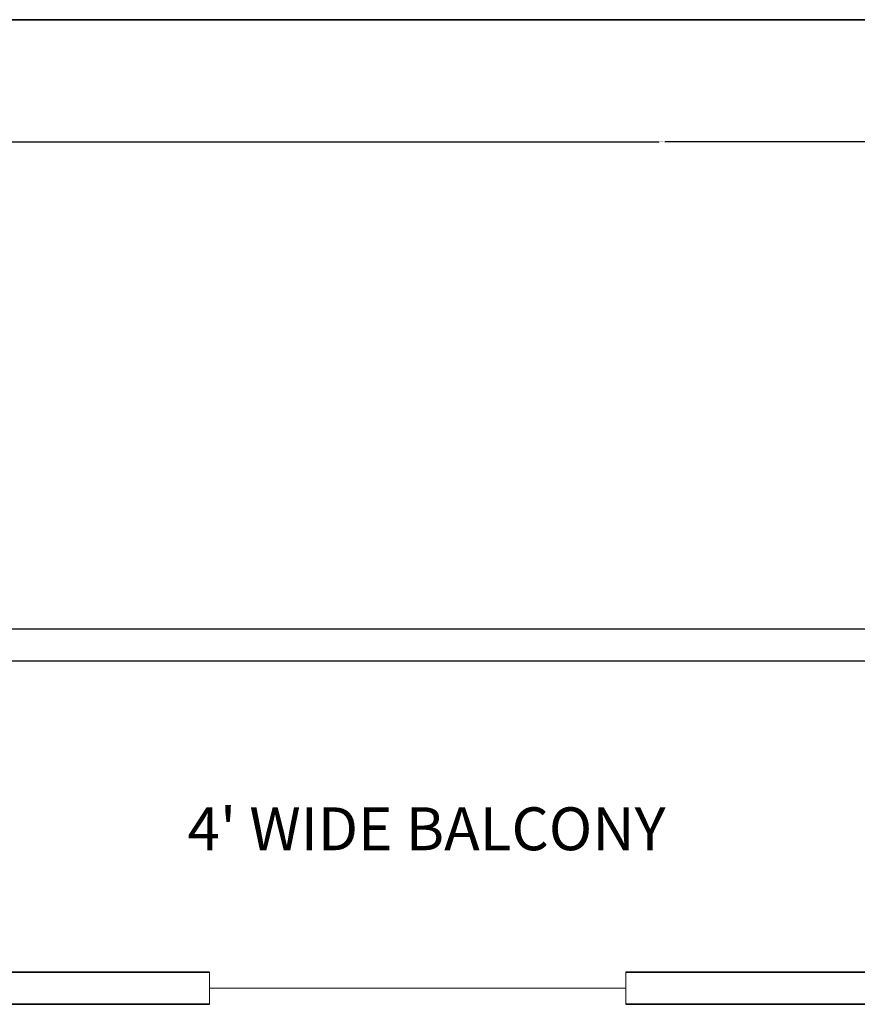
# Model space of a CAD drawing. Units: inches. Extents: x 1088 to 1703, y 668 to 1875.
# Tile 23 of 45: x 1319 to 1436, y 1737 to 1875. Entities that reach past the tile are written whole.
import ezdxf

# ---------------------------------------------------------------- set-up
doc = ezdxf.new("R2010")
doc.units = ezdxf.units.IN
for name, color, linetype, lineweight in [('A-ANNO-DIMS', 2, 'Continuous', 18), ('A-ANNO-TTLB', 7, 'Continuous', 35), ('A-AREA-IDEN', 7, 'Continuous', 18), ('A-DOOR', 4, 'Continuous', 18), ('A-FLOR-HRAL', 7, 'Continuous', 25), ('A-WALL', 7, 'Continuous', 35)]:
    doc.layers.add(name, color=color, linetype=linetype, lineweight=lineweight)
doc.styles.get("Standard").update_dxf_attribs({"font": 'arial.ttf'})
doc.dimstyles.get("Standard").update_dxf_attribs({"dimtxt": 0.18, "dimasz": 0.18, "dimexe": 0.18, "dimexo": 0.0625, "dimgap": 0.09, "dimtad": 0, "dimtih": 1, "dimtoh": 1, "dimdec": 4, "dimzin": 0, "dimdsep": 46, "dimtxsty": 'Standard', "dimcen": 0.09, "dimadec": 0, "dimazin": 0, "dimtfac": 1, "dimtdec": 4, "dimtofl": 0, "dimtmove": 0, "dimatfit": 3, "dimfxl": 1, "dimtolj": 1, "dimtzin": 0, "dimarcsym": 0})

# ---------------------------------------------------------------- blocks, each defined once
blk = doc.blocks.new('*D28')
at = {"layer": 'A-ANNO-DIMS', "color": 0, "lineweight": -2, "transparency": 16777216}
for p, q in [((1170.34, 1803.62), (1170.34, 1857.79)), ((1170.52, 1857.61), (1408.15, 1857.61)), ((1646.56, 1857.61), (1408.94, 1857.61)), ((1646.74, 1745.55), (1646.74, 1857.79))]:
    blk.add_line(p, q, dxfattribs=at)
at = {"layer": 'A-ANNO-DIMS', "color": 0, "transparency": 16777216}
for points in [[(1170.52, 1857.64), (1170.52, 1857.58), (1170.34, 1857.61)], [(1646.56, 1857.64), (1646.56, 1857.58), (1646.74, 1857.61)]]:
    blk.add_solid(points, dxfattribs=at)
at = {"layer": 'Defpoints', "color": 0, "transparency": 16777216}
for p in [(1646.74, 1857.61), (1170.34, 1803.56), (1646.74, 1745.49)]:
    blk.add_point(p, dxfattribs=at)
at = {"layer": 'A-ANNO-DIMS', "color": 0, "transparency": 16777216, "insert": (1408.54, 1857.61), "char_height": 0.18, "attachment_point": 5}
blk.add_mtext('\\A1;476.4', dxfattribs=at)

msp = doc.modelspace()

# ---------------------------------------------------------------- linework, layer by layer
at = {"layer": 'A-ANNO-TTLB'}
msp.add_lwpolyline([(1088.369, 1874.677), (1703.181, 1874.677), (1703.181, 667.947), (1088.369, 667.947)], close=True, dxfattribs=at)
at = {"layer": 'A-DOOR'}
for p, q in [((1345.231, 1741.507), (1345.231, 1737.007)), ((1403.489, 1741.507), (1403.489, 1737.007)), ((1403.489, 1739.257), (1345.231, 1739.257))]:
    msp.add_line(p, q, dxfattribs=at)
at = {"layer": 'A-FLOR-HRAL'}
for p, q in [((1317.345, 1789.507), (1437.345, 1789.507)), ((1437.345, 1785.007), (1317.345, 1785.007))]:
    msp.add_line(p, q, dxfattribs=at)
at = {"layer": 'A-WALL'}
for p, q in [((1345.231, 1741.507), (1317.345, 1741.507)), ((1437.345, 1741.507), (1403.489, 1741.507)), ((1317.345, 1737.007), (1345.231, 1737.007)), ((1403.489, 1737.007), (1437.345, 1737.007))]:
    msp.add_line(p, q, dxfattribs=at)

# ---------------------------------------------------------------- texts
at = {"layer": 'A-AREA-IDEN', "insert": (1342.154, 1764.548), "char_height": 6, "attachment_point": 1}
msp.add_mtext_dynamic_manual_height_columns("4' WIDE BALCONY", width=135.65931, gutter_width=12.5, heights=[0], dxfattribs=at)

# ---------------------------------------------------------------- dimensions: what is measured, and where the dimension line sits
at = {"layer": 'A-ANNO-DIMS'}
dim = msp.add_linear_dim(base=(1646.743, 1857.608), p1=(1170.345, 1803.558), p2=(1646.743, 1745.49), dimstyle='Standard', override={"dimdec": 1, "dimlfac": 1, "dimrnd": 0, "dimzin": 0, "dimdsep": 46, "dimlunit": 2}, dxfattribs=at)
dim.commit()
dim.dimension.update_dxf_attribs({"geometry": '*D28', "text_midpoint": (1408.544, 1857.608)})

doc.saveas('drawing.dxf')
